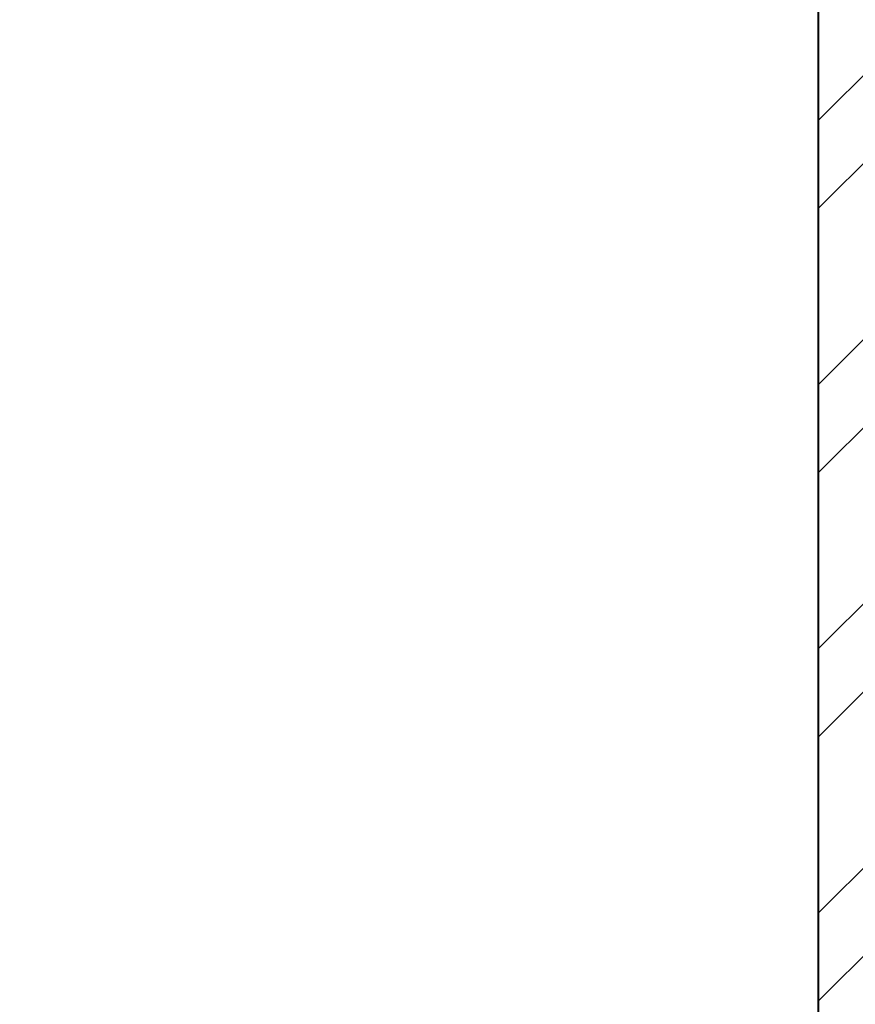
# Model space of a CAD drawing. Units: inches. Extents: x 2063 to 2617, y 1299 to 2210.
# Tile 19 of 22: x 2432 to 2475, y 1889 to 1939. Entities that reach past the tile are written whole.
import ezdxf

# ---------------------------------------------------------------- set-up
doc = ezdxf.new("R2010")
doc.units = ezdxf.units.IN
doc.layers.add('A-WALL', color=7, linetype='Continuous', lineweight=40)
doc.layers.add('A-WALL-PATT', color=215, linetype='Continuous', lineweight=13, true_color=0xa953a0)

msp = doc.modelspace()

# ---------------------------------------------------------------- hatches: boundary and pattern name
at = {"layer": 'A-WALL-PATT'}
h = msp.add_hatch(dxfattribs=at)
h.set_pattern_fill('ANSI32', color=256)
h.paths.add_polyline_path([(2553.6442, 2128.8122), (2511.1703, 2128.8122), (2511.1703, 2124.3122), (2549.1442, 2124.3122), (2549.1442, 2095.662), (2553.6442, 2095.662)])
h.paths.add_polyline_path([(2553.6442, 2035.662), (2549.1442, 2035.662), (2549.1442, 1980.3122), (2503.7214, 1980.3122), (2503.7214, 1975.8122), (2549.1442, 1975.8122), (2549.1442, 1962.9693), (2553.6442, 1962.9693)])
h.paths.add_polyline_path([(2553.6442, 1938.9693), (2549.1442, 1938.9693), (2549.1442, 1927.8122), (2477.1442, 1927.8122), (2477.1442, 1975.8122), (2481.2918, 1975.8122), (2481.2918, 1980.3122), (2453.2648, 1980.3122), (2453.2648, 1975.8122), (2472.6442, 1975.8122), (2472.6442, 1868.3122), (2400.6442, 1868.3122), (2400.6442, 1861.3782), (2405.1442, 1861.3782), (2405.1442, 1863.8122), (2480.9699, 1863.8122), (2480.9699, 1866.0622), (2480.9699, 1868.3122), (2477.1442, 1868.3122), (2477.1442, 1923.3122), (2549.1442, 1923.3122), (2549.1442, 1908.8504), (2553.6442, 1908.8504)])
h.paths.add_polyline_path([(2553.6442, 1884.8504), (2549.1442, 1884.8504), (2549.1442, 1868.3122), (2501.0636, 1868.3122), (2501.0636, 1863.8122), (2549.1442, 1863.8122), (2549.1442, 1826.0298), (2553.6442, 1826.0298)])
h.paths.add_polyline_path([(2388.1504, 1980.3122), (2340.6442, 1980.3122), (2340.6442, 2124.3122), (2358.7501, 2124.3122), (2358.7501, 2128.8122), (2316.3482, 2128.8122), (2316.3482, 2124.3122), (2336.1442, 2124.3122), (2336.1442, 1980.3122), (2289.1737, 1980.3122), (2289.1737, 1975.8122), (2336.1442, 1975.8122), (2336.1442, 1619.3122), (2333.1433, 1619.3122), (2333.1433, 1614.8122), (2344.1671, 1614.8122), (2344.1671, 1617.0622), (2344.1671, 1619.3122), (2340.6442, 1619.3122), (2340.6442, 1975.8122), (2388.1504, 1975.8122), (2388.1504, 1978.0622)])
h.paths.add_polyline_path([(2290.1442, 1614.8122), (2301.4594, 1614.8122), (2301.4594, 1617.0622), (2301.4594, 1619.3122), (2285.6442, 1619.3122), (2285.6442, 1566.8122), (2280.8619, 1566.8122), (2280.8619, 1564.5622), (2280.8619, 1562.3122), (2285.6442, 1562.3122), (2285.6442, 1442.3122), (2281.7879, 1442.3122), (2281.7879, 1437.8122), (2285.6442, 1437.8122), (2285.6442, 1401.8122), (2290.1442, 1401.8122)])
h.paths.add_polyline_path([(2549.1442, 1731.8122), (2405.1442, 1731.8122), (2405.1442, 1834.4638), (2402.8942, 1834.4638), (2400.6442, 1834.4638), (2400.6442, 1727.3122), (2549.1442, 1727.3122)])
h.paths.add_polyline_path([(2553.6442, 1766.0298), (2551.3942, 1766.0298), (2549.1442, 1766.0298), (2549.1442, 1686.7767), (2553.6442, 1686.7767)])
h.paths.add_polyline_path([(2553.6442, 1638.7767), (2551.3942, 1638.7767), (2549.1442, 1638.7767), (2549.1442, 1619.3122), (2448.6442, 1619.3122), (2448.6442, 1610.5671), (2450.8942, 1610.5671), (2453.1442, 1610.5671), (2453.1442, 1614.8122), (2549.1442, 1614.8122), (2549.1442, 1601.6421), (2553.6442, 1601.6421)])
h.paths.add_polyline_path([(2553.6442, 1577.6421), (2551.3942, 1577.6421), (2549.1442, 1577.6421), (2549.1442, 1566.8122), (2453.1442, 1566.8122), (2453.1442, 1591.5045), (2451.0335, 1591.5045), (2448.6442, 1591.5045), (2448.6442, 1566.8122), (2434.0475, 1566.8122), (2434.0475, 1562.3122), (2549.1442, 1562.3122), (2549.1442, 1533.48), (2553.6442, 1533.48)])
h.paths.add_polyline_path([(2553.6442, 1473.48), (2549.1442, 1473.48), (2549.1442, 1442.3122), (2502.6258, 1442.3122), (2502.6258, 1437.8122), (2549.1442, 1437.8122), (2549.1442, 1401.8122), (2553.6442, 1401.8122)])
h.paths.add_polyline_path([(2395.6442, 1562.3122), (2400.0901, 1562.3122), (2400.0901, 1564.5622), (2400.0901, 1566.8122), (2395.6442, 1566.8122), (2395.6442, 1619.3122), (2379.1127, 1619.3122), (2379.1127, 1614.8122), (2391.1442, 1614.8122), (2391.1442, 1401.8122), (2395.6442, 1401.8122), (2395.6442, 1437.8122), (2399.2425, 1437.8122), (2399.2425, 1440.0622), (2399.2425, 1442.3122), (2395.6442, 1442.3122)])
h.paths.add_polyline_path([(2442.6258, 1442.3122), (2419.6262, 1442.3122), (2419.6262, 1437.8122), (2442.6258, 1437.8122), (2442.6258, 1440.0622)])
h.paths.add_polyline_path([(2127.6442, 1480.2532), (2125.3942, 1480.2532), (2123.1442, 1480.2532), (2123.1442, 1401.8122), (2127.6442, 1401.8122), (2127.6442, 1437.8122), (2145.1538, 1437.8122), (2145.1538, 1440.0622), (2145.1538, 1442.3122), (2127.6442, 1442.3122)])
h.paths.add_polyline_path([(2259.809, 1442.3122), (2205.1538, 1442.3122), (2205.1538, 1437.8122), (2259.809, 1437.8122), (2259.809, 1440.0622)])
h.paths.add_polyline_path([(2127.6442, 1659.7652), (2123.1442, 1659.7652), (2123.1442, 1605.5161), (2125.3942, 1605.5161), (2127.6442, 1605.5161), (2127.6442, 1614.8122), (2223.6442, 1614.8122), (2223.6442, 1611.2723), (2228.1442, 1611.2723), (2228.1442, 1619.3122), (2127.6442, 1619.3122)])
h.paths.add_polyline_path([(2244.8673, 1566.8122), (2228.1442, 1566.8122), (2228.1442, 1590.8122), (2225.8942, 1590.8122), (2223.6442, 1590.8122), (2223.6442, 1566.8122), (2127.6442, 1566.8122), (2127.6442, 1581.5161), (2123.1442, 1581.5161), (2123.1442, 1540.2532), (2127.6442, 1540.2532), (2127.6442, 1562.3122), (2244.8673, 1562.3122), (2244.8673, 1564.5622)])
h.paths.add_polyline_path([(2172.5174, 1868.3122), (2127.6442, 1868.3122), (2127.6442, 1886.5833), (2123.1442, 1886.5833), (2123.1442, 1832.6633), (2127.6442, 1832.6633), (2127.6442, 1863.8122), (2172.5174, 1863.8122), (2172.5174, 1866.0622)])
h.paths.add_polyline_path([(2276.1442, 1868.3122), (2204.1442, 1868.3122), (2204.1442, 1923.3122), (2204.1442, 1975.8122), (2224.8362, 1975.8122), (2224.8362, 1978.1097), (2224.8362, 1980.3122), (2195.0729, 1980.3122), (2195.0729, 1978.0622), (2195.0729, 1975.8122), (2199.6442, 1975.8122), (2199.6442, 1927.8122), (2127.6442, 1927.8122), (2127.6442, 1942.3492), (2123.1442, 1942.3492), (2123.1442, 1910.5833), (2127.6442, 1910.5833), (2127.6442, 1923.3122), (2199.6442, 1923.3122), (2199.6442, 1868.3122), (2194.8228, 1868.3122), (2194.8228, 1864.7337), (2194.8228, 1863.8122), (2271.6442, 1863.8122), (2271.6442, 1860.0507), (2276.1442, 1860.0507)])
h.paths.add_polyline_path([(2276.1442, 1829.994), (2273.8942, 1829.994), (2271.6442, 1829.994), (2271.6442, 1731.8122), (2127.6442, 1731.8122), (2127.6442, 1772.6633), (2123.1442, 1772.6633), (2123.1442, 1707.7652), (2127.6442, 1707.7652), (2127.6442, 1727.3122), (2276.1442, 1727.3122)])
h.paths.add_polyline_path([(2127.6442, 2022.1152), (2123.1442, 2022.1152), (2123.1442, 1966.3492), (2127.6442, 1966.3492), (2127.6442, 1975.8122), (2174.2082, 1975.8122), (2174.2082, 1978.0622), (2174.2082, 1980.3122), (2127.6442, 1980.3122)])
h.paths.add_polyline_path([(2361.9755, 1678.588), (2398.4558, 1678.588), (2398.4558, 1697.2453), (2361.9755, 1697.2453)], flags=9)
h.paths.add_polyline_path([(2351.5397, 1780.4072), (2386.1987, 1780.4072), (2386.1987, 1790.7107), (2351.5397, 1790.7107)], flags=25)
h.paths.add_polyline_path([(2350.6753, 1940.9321), (2387.6024, 1940.9321), (2387.6024, 1959.5894), (2350.6753, 1959.5894)], flags=25)
h.paths.add_polyline_path([(2254.9545, 1684.638), (2295.0943, 1684.638), (2295.0943, 1703.2953), (2254.9545, 1703.2953)], flags=9)
h.paths.add_polyline_path([(2282.4946, 1782.4438), (2317.1535, 1782.4438), (2317.1535, 1792.7474), (2282.4946, 1792.7474)], flags=9)
h.paths.add_polyline_path([(2270.327, 1939.2854), (2307.254, 1939.2854), (2307.254, 1957.9428), (2270.327, 1957.9428)], flags=9)

# ---------------------------------------------------------------- linework, layer by layer
at = {"layer": 'A-WALL'}
msp.add_line((2472.6442, 1975.8122), (2472.6442, 1868.3122), dxfattribs=at)

doc.saveas('drawing.dxf')
